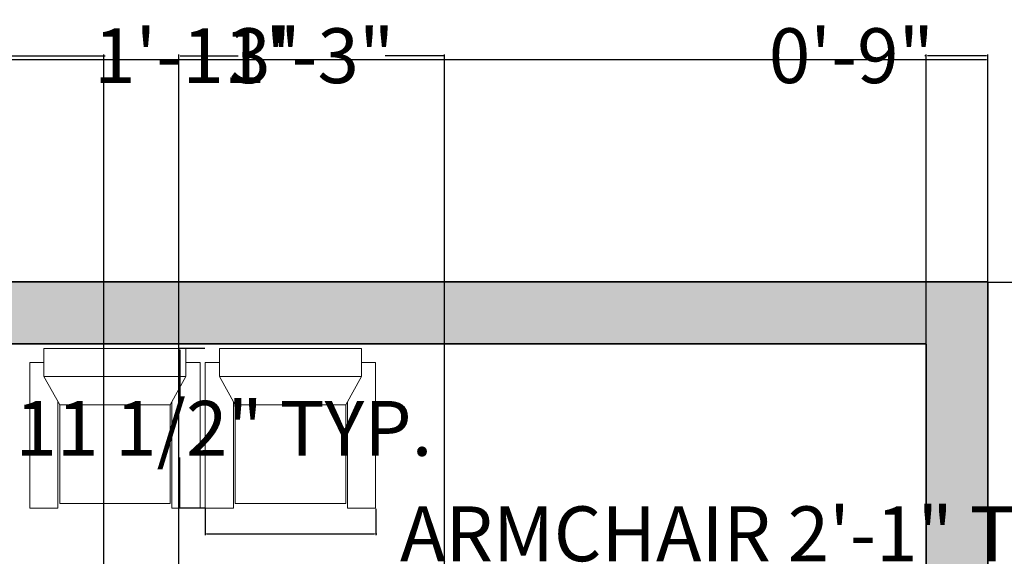
# Model space of a CAD drawing. Units: inches. Extents: x -4737294 to -4736756, y 1716389 to 1717040.
# Tile 24 of 25: x -4736996 to -4736853, y 1716962 to 1717040. Entities that reach past the tile are written whole.
import ezdxf

# ---------------------------------------------------------------- set-up
doc = ezdxf.new("R2010")
doc.units = ezdxf.units.IN
doc.header["$MEASUREMENT"] = 0
for name, color, linetype, lineweight in [('A-ANNO-DIMS', 2, 'Continuous', 18), ('A-WALL-PATT', 244, 'Continuous', 13), ('furniture', 250, 'Continuous', 18), ('walls', 252, 'Continuous', 35)]:
    doc.layers.add(name, color=color, linetype=linetype, lineweight=lineweight)
doc.styles.get("Standard").update_dxf_attribs({"font": 'arial.ttf'})
doc.dimstyles.get("Standard").update_dxf_attribs({"dimtxt": 8, "dimasz": 0.18, "dimexe": 0.18, "dimexo": 0.0625, "dimgap": 0.09, "dimtad": 0, "dimtih": 1, "dimtoh": 1, "dimzin": 0, "dimdsep": 46, "dimlunit": 3, "dimtxsty": 'Standard', "dimcen": 0.09, "dimadec": 0, "dimazin": 0, "dimtfac": 1, "dimtofl": 0, "dimtmove": 0, "dimatfit": 3, "dimfxl": 1, "dimtolj": 1, "dimtzin": 0, "dimarcsym": 0})

# ---------------------------------------------------------------- blocks, each defined once
blk = doc.blocks.new('*D21')
at = {"layer": 'A-ANNO-DIMS', "color": 0, "lineweight": -2, "transparency": 16777216}
for p, q in [((-4737215.14, 1717002.13), (-4737215.14, 1717034.64)), ((-4737214.96, 1717034.46), (-4737042.02, 1717034.46)), ((-4736855.32, 1717034.46), (-4737028.27, 1717034.46)), ((-4736855.14, 1717002.13), (-4736855.14, 1717034.64))]:
    blk.add_line(p, q, dxfattribs=at)
at = {"layer": 'A-ANNO-DIMS', "color": 0, "transparency": 16777216}
for points in [[(-4737214.96, 1717034.49), (-4737214.96, 1717034.43), (-4737215.14, 1717034.46)], [(-4736855.32, 1717034.49), (-4736855.32, 1717034.43), (-4736855.14, 1717034.46)]]:
    blk.add_solid(points, dxfattribs=at)
at = {"layer": 'Defpoints', "color": 0, "transparency": 16777216}
for p in [(-4736855.14, 1717034.46), (-4737215.14, 1717002.06), (-4736855.14, 1717002.06)]:
    blk.add_point(p, dxfattribs=at)
at = {"layer": 'A-ANNO-DIMS', "color": 0, "transparency": 16777216, "insert": (-4737035.14, 1717034.46), "char_height": 8, "attachment_point": 5}
blk.add_mtext("\\A1;30'", dxfattribs=at)
blk = doc.blocks.new('*D22')
at = {"layer": 'A-ANNO-DIMS', "color": 0, "lineweight": -2, "transparency": 16777216}
for p, q in [((-4736855.08, 1717002.06), (-4736830.06, 1717002.06)), ((-4736830.24, 1717001.88), (-4736830.24, 1716736.22)), ((-4736830.24, 1716462.24), (-4736830.24, 1716727.91)), ((-4736855.08, 1716462.06), (-4736830.06, 1716462.06))]:
    blk.add_line(p, q, dxfattribs=at)
at = {"layer": 'A-ANNO-DIMS', "color": 0, "transparency": 16777216}
for points in [[(-4736830.27, 1717001.88), (-4736830.21, 1717001.88), (-4736830.24, 1717002.06)], [(-4736830.27, 1716462.24), (-4736830.21, 1716462.24), (-4736830.24, 1716462.06)]]:
    blk.add_solid(points, dxfattribs=at)
at = {"layer": 'Defpoints', "color": 0, "transparency": 16777216}
for p in [(-4736855.14, 1717002.06), (-4736830.24, 1717002.06), (-4736855.14, 1716462.06)]:
    blk.add_point(p, dxfattribs=at)
at = {"layer": 'A-ANNO-DIMS', "color": 0, "transparency": 16777216, "insert": (-4736830.24, 1716732.06), "char_height": 8, "attachment_point": 5}
blk.add_mtext("\\A1;45'", dxfattribs=at)
blk = doc.blocks.new('FABRIC SOFA 1S')
at = {"layer": 'furniture'}
for p, q in [((3, 18.12), (34, 18.12)), ((3, 15.12), (3, 18.12)), ((34, 12.12), (34, 18.12)), ((0, -15.12), (0, 15.12)), ((6, 15.12), (0, 15.12)), ((6, -15.12), (6, 15.12)), ((12, 11.75), (6, 15.12)), ((11.33, 12.12), (34, 12.12)), ((6, -15.12), (12, -11.75)), ((11.33, -12.12), (34, -12.12)), ((34, -12.12), (34, -18.12)), ((6, -15.12), (0, -15.12)), ((3, -18.12), (3, -15.12)), ((3, -18.12), (34, -18.12))]:
    blk.add_line(p, q, dxfattribs=at)
blk.add_lwpolyline([(12, -11.75), (12, 11.75), (33, 11.75), (33, -11.75)], close=True, dxfattribs=at)
blk = doc.blocks.new('*D27')
at = {"layer": 'A-ANNO-DIMS', "color": 0, "lineweight": -2, "transparency": 16777216}
for p, q in [((-4736969.31, 1716969), (-4736969.31, 1716965.16)), ((-4736944.45, 1716969), (-4736944.45, 1716965.16)), ((-4736969.13, 1716965.34), (-4736944.63, 1716965.34)), ((-4736944.45, 1716965.34), (-4736944.27, 1716965.34))]:
    blk.add_line(p, q, dxfattribs=at)
at = {"layer": 'A-ANNO-DIMS', "color": 0, "transparency": 16777216}
for points in [[(-4736969.13, 1716965.37), (-4736969.13, 1716965.31), (-4736969.31, 1716965.34)], [(-4736944.63, 1716965.37), (-4736944.63, 1716965.31), (-4736944.45, 1716965.34)]]:
    blk.add_solid(points, dxfattribs=at)
at = {"layer": 'Defpoints', "color": 0, "transparency": 16777216}
for p in [(-4736969.31, 1716969.06), (-4736944.45, 1716969.06), (-4736944.45, 1716965.34)]:
    blk.add_point(p, dxfattribs=at)
at = {"layer": 'A-ANNO-DIMS', "color": 0, "transparency": 16777216, "insert": (-4736888.21, 1716965.34), "char_height": 8, "attachment_point": 5}
blk.add_mtext('\\A1;ARMCHAIR 2\'-1" TYP.', dxfattribs=at)
blk = doc.blocks.new('*D28')
at = {"layer": 'A-ANNO-DIMS', "color": 0, "lineweight": -2, "transparency": 16777216}
for p, q in [((-4736969.37, 1716992.37), (-4736973.21, 1716992.37)), ((-4736973.03, 1716992.19), (-4736973.03, 1716984.95)), ((-4736973.03, 1716969.24), (-4736973.03, 1716976.49)), ((-4736969.37, 1716969.06), (-4736973.21, 1716969.06))]:
    blk.add_line(p, q, dxfattribs=at)
at = {"layer": 'A-ANNO-DIMS', "color": 0, "transparency": 16777216}
for points in [[(-4736973.06, 1716992.19), (-4736973, 1716992.19), (-4736973.03, 1716992.37)], [(-4736973.06, 1716969.24), (-4736973, 1716969.24), (-4736973.03, 1716969.06)]]:
    blk.add_solid(points, dxfattribs=at)
at = {"layer": 'Defpoints', "color": 0, "transparency": 16777216}
for p in [(-4736969.31, 1716992.37), (-4736973.03, 1716969.06), (-4736969.31, 1716969.06)]:
    blk.add_point(p, dxfattribs=at)
at = {"layer": 'A-ANNO-DIMS', "color": 0, "transparency": 16777216, "insert": (-4736973.03, 1716980.72), "char_height": 8, "attachment_point": 5}
blk.add_mtext('\\A1;1\'-11 1/2" TYP.', dxfattribs=at)
blk = doc.blocks.new('*D61')
at = {"layer": 'A-ANNO-DIMS', "color": 0, "lineweight": -2, "transparency": 16777216}
for p, q in [((-4736864.144166, 1716993.127125), (-4736864.144166, 1717035.244625)), ((-4736855.144166, 1717002.127125), (-4736855.144166, 1717035.244625)), ((-4736864.144166, 1717035.064625), (-4736864.324166, 1717035.064625)), ((-4736855.324166, 1717035.064625), (-4736863.964166, 1717035.064625))]:
    blk.add_line(p, q, dxfattribs=at)
at = {"layer": 'A-ANNO-DIMS', "color": 0, "transparency": 16777216}
for points in [[(-4736863.964166, 1717035.094625), (-4736863.964166, 1717035.034625), (-4736864.144166, 1717035.064625)], [(-4736855.324166, 1717035.094625), (-4736855.324166, 1717035.034625), (-4736855.144166, 1717035.064625)]]:
    blk.add_solid(points, dxfattribs=at)
at = {"layer": 'Defpoints', "color": 0, "transparency": 16777216}
for p in [(-4736864.144166, 1717035.064625), (-4736855.144166, 1717002.064625), (-4736864.144166, 1716993.064625)]:
    blk.add_point(p, dxfattribs=at)
at = {"layer": 'A-ANNO-DIMS', "color": 0, "transparency": 16777216, "insert": (-4736875.047181, 1717035.064625), "char_height": 8, "attachment_point": 5}
blk.add_mtext('\\A1;0\'-9"', dxfattribs=at)
blk = doc.blocks.new('*D65')
at = {"layer": 'A-ANNO-DIMS', "color": 0, "lineweight": -2, "transparency": 16777216}
for p, q in [((-4737007.1, 1716596.13), (-4737007.1, 1717035.24)), ((-4736984.09, 1716596.13), (-4736984.09, 1717035.24)), ((-4737006.92, 1717035.06), (-4736984.27, 1717035.06)), ((-4736984.09, 1717035.06), (-4736983.91, 1717035.06))]:
    blk.add_line(p, q, dxfattribs=at)
at = {"layer": 'A-ANNO-DIMS', "color": 0, "transparency": 16777216}
for points in [[(-4737006.92, 1717035.09), (-4737006.92, 1717035.03), (-4737007.1, 1717035.06)], [(-4736984.27, 1717035.09), (-4736984.27, 1717035.03), (-4736984.09, 1717035.06)]]:
    blk.add_solid(points, dxfattribs=at)
at = {"layer": 'Defpoints', "color": 0, "transparency": 16777216}
for p in [(-4736984.09, 1717035.06), (-4737007.1, 1716596.06), (-4736984.09, 1716596.06)]:
    blk.add_point(p, dxfattribs=at)
at = {"layer": 'A-ANNO-DIMS', "color": 0, "transparency": 16777216, "insert": (-4736970.46, 1717035.06), "char_height": 8, "attachment_point": 5}
blk.add_mtext('\\A1;1\'-11"', dxfattribs=at)
blk = doc.blocks.new('*D66')
at = {"layer": 'A-ANNO-DIMS', "color": 0, "lineweight": -2, "transparency": 16777216}
for p, q in [((-4736973.14, 1716668.63), (-4736973.14, 1717035.24)), ((-4736934.39, 1716668.63), (-4736934.39, 1717035.24)), ((-4736972.96, 1717035.06), (-4736964.49, 1717035.06)), ((-4736934.57, 1717035.06), (-4736943.05, 1717035.06))]:
    blk.add_line(p, q, dxfattribs=at)
at = {"layer": 'A-ANNO-DIMS', "color": 0, "transparency": 16777216}
for points in [[(-4736972.96, 1717035.09), (-4736972.96, 1717035.03), (-4736973.14, 1717035.06)], [(-4736934.57, 1717035.09), (-4736934.57, 1717035.03), (-4736934.39, 1717035.06)]]:
    blk.add_solid(points, dxfattribs=at)
at = {"layer": 'Defpoints', "color": 0, "transparency": 16777216}
for p in [(-4736934.39, 1717035.06), (-4736973.14, 1716668.56), (-4736934.39, 1716668.56)]:
    blk.add_point(p, dxfattribs=at)
at = {"layer": 'A-ANNO-DIMS', "color": 0, "transparency": 16777216, "insert": (-4736953.77, 1717035.06), "char_height": 8, "attachment_point": 5}
blk.add_mtext('\\A1;3\'-3"', dxfattribs=at)

msp = doc.modelspace()

# ---------------------------------------------------------------- hatches: boundary and pattern name
at = {"layer": 'A-WALL-PATT'}
h = msp.add_hatch(color=256, dxfattribs=at)
h.dxf.hatch_style = 1
h.paths.add_polyline_path([(-4737206.144, 1716844.565), (-4737110.144, 1716844.565), (-4737110.144, 1716823.907), (-4737105.644, 1716823.907), (-4737105.644, 1716844.565), (-4737098.44, 1716844.565), (-4737098.44, 1716849.065), (-4737206.144, 1716849.065), (-4737206.144, 1716993.065), (-4736864.144, 1716993.065), (-4736864.144, 1716849.065), (-4736963.275, 1716849.065), (-4736994.446, 1716849.065), (-4736997.144, 1716849.065), (-4736997.144, 1716844.565), (-4736864.144, 1716844.565), (-4736864.144, 1716668.565), (-4736934.391, 1716668.565), (-4736934.391, 1716664.065), (-4736864.144, 1716664.065), (-4736864.144, 1716462.065), (-4736855.144, 1716462.065), (-4736855.144, 1717002.065), (-4737215.144, 1717002.065), (-4737215.144, 1716462.065), (-4737206.144, 1716462.065), (-4737206.144, 1716659.065), (-4737062.144, 1716659.065), (-4737062.144, 1716647.493), (-4737057.644, 1716647.493), (-4737057.644, 1716796.565), (-4737071.812, 1716796.565), (-4737071.812, 1716792.065), (-4737070.805, 1716792.065), (-4737062.144, 1716792.065), (-4737062.144, 1716668.065), (-4737206.144, 1716668.065), (-4737206.144, 1716792.065), (-4737093.784, 1716792.065), (-4737093.784, 1716796.565), (-4737206.144, 1716796.565)])

# ---------------------------------------------------------------- linework, layer by layer
at = {"layer": 'walls'}
for p, q in [((-4737215.144, 1717002.065), (-4736855.144, 1717002.065)), ((-4736855.144, 1717002.065), (-4736855.144, 1716462.065)), ((-4737206.144, 1716993.065), (-4736864.144, 1716993.065)), ((-4736864.144, 1716993.065), (-4736864.144, 1716849.065))]:
    msp.add_line(p, q, dxfattribs=at)

# ---------------------------------------------------------------- block references
at = {"layer": 'furniture', "xscale": 0.685544738852578, "yscale": 0.685544738852578, "zscale": 0.685544738852578, "rotation": 270}
for p in [(-4736982.488, 1716992.373), (-4736956.88, 1716992.373)]:
    msp.add_blockref('FABRIC SOFA 1S', p, dxfattribs=at)

# ---------------------------------------------------------------- dimensions: what is measured, and where the dimension line sits
at = {"layer": 'A-ANNO-DIMS'}
for base, p1, p2, override, picture, middle in [((-4736855.144, 1717034.458), (-4737215.144, 1717002.065), (-4736855.144, 1717002.065), {"dimclrd": 0, "dimclre": 0, "dimclrt": 0}, '*D21', (-4737035.144, 1717034.458)), ((-4736984.094, 1717035.065), (-4737007.097, 1716596.065), (-4736984.094, 1716596.065), {"dimdec": 1, "dimlfac": 1, "dimrnd": 0, "dimzin": 1, "dimdsep": 46, "dimlunit": 4, "dimfrac": 2}, '*D65', (-4736970.46, 1717035.065)), ((-4736934.391, 1717035.065), (-4736973.144, 1716668.565), (-4736934.391, 1716668.565), {"dimdec": 1, "dimlfac": 1, "dimrnd": 0, "dimzin": 1, "dimdsep": 46, "dimlunit": 4, "dimfrac": 2}, '*D66', (-4736953.768, 1717035.065)), ((-4736864.144, 1717035.065), (-4736855.144, 1717002.065), (-4736864.144, 1716993.065), {"dimdec": 1, "dimlfac": 1, "dimrnd": 0, "dimzin": 1, "dimdsep": 46, "dimlunit": 4, "dimfrac": 2}, '*D61', (-4736875.047, 1717035.065))]:
    dim = msp.add_linear_dim(base=base, p1=p1, p2=p2, dimstyle='Standard', override=override, dxfattribs=at)
    dim.commit()
    dim.dimension.update_dxf_attribs({"geometry": picture, "text_midpoint": middle})
dim = msp.add_linear_dim(base=(-4736830.238, 1717002.065), p1=(-4736855.144, 1716462.065), p2=(-4736855.144, 1717002.065), angle=90, dimstyle='Standard', override={"dimclrd": 0, "dimclre": 0, "dimclrt": 0}, dxfattribs=at)
dim.commit()
dim.dimension.update_dxf_attribs({"geometry": '*D22', "text_midpoint": (-4736830.238, 1716732.065)})
dim = msp.add_linear_dim(base=(-4736973.033, 1716969.065), p1=(-4736969.306, 1716992.373), p2=(-4736969.306, 1716969.065), angle=270, text='<> TYP.', dimstyle='Standard', override={"dimdec": 1, "dimlfac": 1, "dimrnd": 0, "dimzin": 1, "dimdsep": 46, "dimlunit": 4, "dimfrac": 2}, dxfattribs=at)
dim.commit()
dim.dimension.update_dxf_attribs({"geometry": '*D28', "text_midpoint": (-4736973.033, 1716980.719)})
dim = msp.add_linear_dim(base=(-4736944.455, 1716965.337), p1=(-4736969.306, 1716969.065), p2=(-4736944.455, 1716969.065), text='ARMCHAIR <> TYP.', dimstyle='Standard', override={"dimdec": 1, "dimlfac": 1, "dimrnd": 0, "dimzin": 1, "dimdsep": 46, "dimlunit": 4, "dimfrac": 2}, dxfattribs=at)
dim.commit()
dim.dimension.update_dxf_attribs({"geometry": '*D27', "text_midpoint": (-4736888.215, 1716965.337)})

doc.saveas('drawing.dxf')
